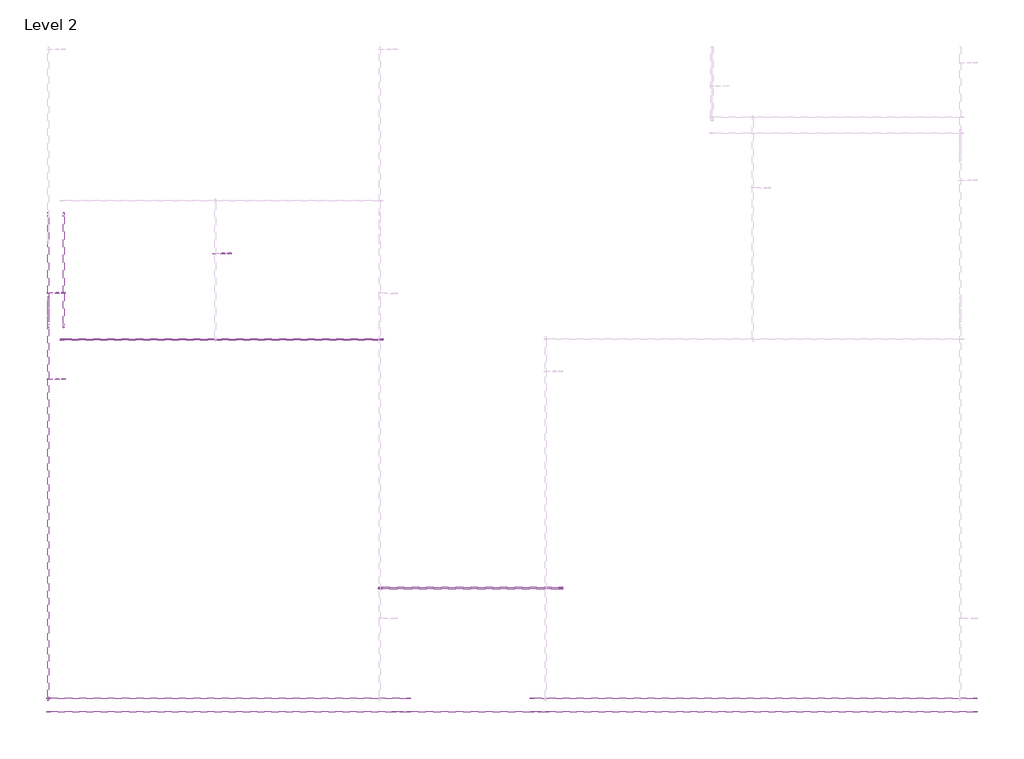
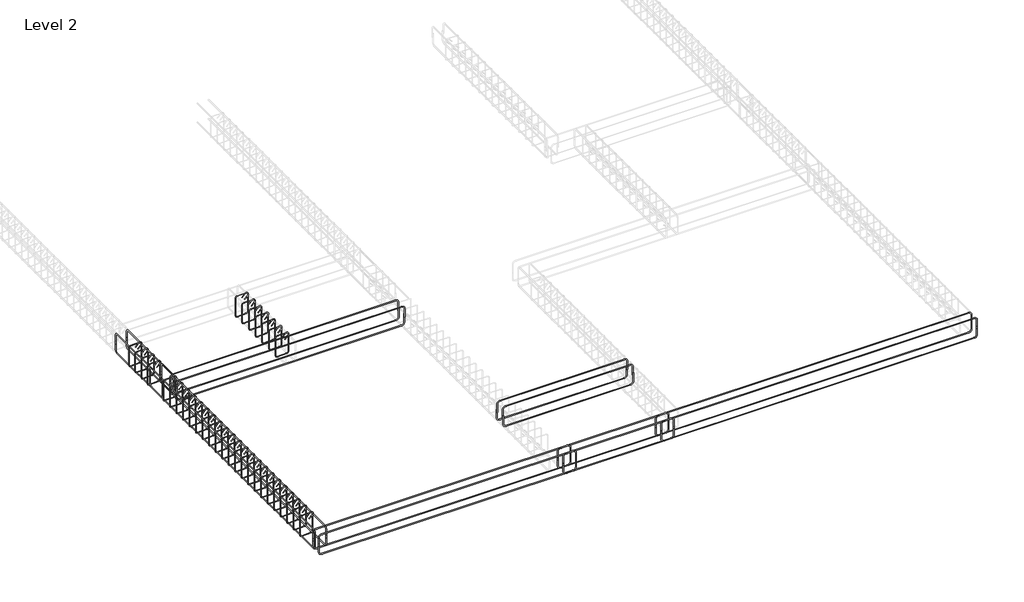
# One storey, part 2 of 5: 17 reinforcing bars.
"""IFC4 building model written with IfcOpenShell, lengths in millimetres."""

from ifc_helpers import new_model, si_unit, point, frame, origin, place, context, project, spatial, polyline, circle_curve, trimmed, segment, composite_curve, source, transform, mapped, element, save
from ifc_brep_helpers import swept_disk

model = new_model("IFC4")

# Units and contexts
model_context = context("Model", 3, world=origin())
ifc_project = project(units=[si_unit("LENGTHUNIT", "METRE", prefix="MILLI")], contexts=[model_context])

# Site, building, storey
site = spatial("IfcSite", under=ifc_project)
building = spatial("IfcBuilding", under=site)
storey = spatial("IfcBuildingStorey", under=building, Name="Level 2", Elevation=3048.0)

# Reinforcing bars
placement = place(None, origin())
reinforcing_bar_shape = source(origin(), model_context, "Body", "SolidModel", [
    swept_disk(composite_curve([segment(polyline([(-15212.455746, 3821.0577522, 5841.8967919), (-15212.455746, 3821.0577522, 5994.2967919)]), True, "CONTINUOUS"), segment(trimmed(circle_curve(frame((-15212.455746, 3776.9887522, 5994.2967919), z_axis=(1.0, 0.0, 0.0), x_axis=(0.0, 44.06899999999996, 0.0)), 44.069), [point((-15212.455746, 3821.0577522, 5994.2967919))], [point((-15212.455746, 3776.9887522, 6038.3657919))], True, "CARTESIAN"), True, "CONTINUOUS"), segment(polyline([(-15212.455746, 3776.9887522, 6038.3657919), (-15212.455746, 2478.6647522, 6038.3657919)]), True, "CONTINUOUS"), segment(trimmed(circle_curve(frame((-15212.455746, 2478.6647522, 5994.2967919), z_axis=(1.0, 0.0, 0.0), x_axis=(0.0, 0.0, 44.068999999999505)), 44.069), [point((-15212.455746, 2478.6647522, 6038.3657919))], [point((-15212.455746, 2434.5957522, 5994.2967919))], True, "CARTESIAN"), True, "CONTINUOUS"), segment(polyline([(-15212.455746, 2434.5957522, 5994.2967919), (-15212.455746, 2434.5957522, 5841.8967919)]), True, "CONTINUOUS")], self_intersect=False), 5.969),
])
element("IfcReinforcingBar", 1, at=placement, inside=storey, context=model_context, shape_type="MappedRepresentation", body=[
    mapped(reinforcing_bar_shape, transform((0.0, 0.0, 0.0), x_axis=(1.0, 0.0, 0.0), y_axis=(0.0, 1.0, 0.0), z_axis=(0.0, 0.0, 1.0))),
    mapped(reinforcing_bar_shape, transform((-189.5315837, 0.0, 0.0), x_axis=(1.0, 0.0, 0.0), y_axis=(0.0, 1.0, 0.0), z_axis=(0.0, 0.0, 1.0))),
])
reinforcing_bar_2_shape = source(origin(), model_context, "Body", "SolidModel", [
    swept_disk(composite_curve([segment(polyline([(-15212.455746, 2434.5957522, 5892.9032081), (-15212.455746, 2434.5957522, 5740.5032081)]), True, "CONTINUOUS"), segment(trimmed(circle_curve(frame((-15212.455746, 2478.6647522, 5740.5032081), z_axis=(1.0, 0.0, 0.0), x_axis=(0.0, -44.06899999999996, 0.0)), 44.069), [point((-15212.455746, 2434.5957522, 5740.5032081))], [point((-15212.455746, 2478.6647522, 5696.4342081))], True, "CARTESIAN"), True, "CONTINUOUS"), segment(polyline([(-15212.455746, 2478.6647522, 5696.4342081), (-15212.455746, 3776.9887522, 5696.4342081)]), True, "CONTINUOUS"), segment(trimmed(circle_curve(frame((-15212.455746, 3776.9887522, 5740.5032081), z_axis=(1.0, 0.0, 0.0), x_axis=(0.0, 0.0, -44.068999999999505)), 44.069), [point((-15212.455746, 3776.9887522, 5696.4342081))], [point((-15212.455746, 3821.0577522, 5740.5032081))], True, "CARTESIAN"), True, "CONTINUOUS"), segment(polyline([(-15212.455746, 3821.0577522, 5740.5032081), (-15212.455746, 3821.0577522, 5892.9032081)]), True, "CONTINUOUS")], self_intersect=False), 5.969),
])
element("IfcReinforcingBar", 2, at=placement, inside=storey, context=model_context, shape_type="MappedRepresentation", body=[
    mapped(reinforcing_bar_2_shape, transform((0.0, 0.0, 0.0), x_axis=(1.0, 0.0, 0.0), y_axis=(0.0, 1.0, 0.0), z_axis=(0.0, 0.0, 1.0))),
    mapped(reinforcing_bar_2_shape, transform((-189.5315837, 0.0, 0.0), x_axis=(1.0, 0.0, 0.0), y_axis=(0.0, 1.0, 0.0), z_axis=(0.0, 0.0, 1.0))),
])
reinforcing_bar_3_shape = source(origin(), model_context, "Body", "SolidModel", [
    swept_disk(composite_curve([segment(polyline([(-15212.455746, 2803.6577522, 5841.8967919), (-15212.455746, 2803.6577522, 5994.2967919)]), True, "CONTINUOUS"), segment(trimmed(circle_curve(frame((-15212.455746, 2759.5887522, 5994.2967919), z_axis=(1.0, 0.0, 0.0), x_axis=(0.0, 44.06899999999996, 0.0)), 44.069), [point((-15212.455746, 2803.6577522, 5994.2967919))], [point((-15212.455746, 2759.5887522, 6038.3657919))], True, "CARTESIAN"), True, "CONTINUOUS"), segment(polyline([(-15212.455746, 2759.5887522, 6038.3657919), (-15212.455746, -2021.3352478, 6038.3657919)]), True, "CONTINUOUS"), segment(trimmed(circle_curve(frame((-15212.455746, -2021.3352478, 5994.2967919), z_axis=(1.0, 0.0, 0.0), x_axis=(0.0, 0.0, 44.068999999999505)), 44.069), [point((-15212.455746, -2021.3352478, 6038.3657919))], [point((-15212.455746, -2065.4042478, 5994.2967919))], True, "CARTESIAN"), True, "CONTINUOUS"), segment(polyline([(-15212.455746, -2065.4042478, 5994.2967919), (-15212.455746, -2065.4042478, 5841.8967919)]), True, "CONTINUOUS")], self_intersect=False), 5.969),
])
element("IfcReinforcingBar", 3, at=placement, inside=storey, context=model_context, shape_type="MappedRepresentation", body=[
    mapped(reinforcing_bar_3_shape, transform((0.0, 0.0, 0.0), x_axis=(1.0, 0.0, 0.0), y_axis=(0.0, 1.0, 0.0), z_axis=(0.0, 0.0, 1.0))),
    mapped(reinforcing_bar_3_shape, transform((-189.5315837, 0.0, 0.0), x_axis=(1.0, 0.0, 0.0), y_axis=(0.0, 1.0, 0.0), z_axis=(0.0, 0.0, 1.0))),
])
reinforcing_bar_4_shape = source(origin(), model_context, "Body", "SolidModel", [
    swept_disk(composite_curve([segment(polyline([(-15212.455746, -2065.4042478, 5892.9032081), (-15212.455746, -2065.4042478, 5740.5032081)]), True, "CONTINUOUS"), segment(trimmed(circle_curve(frame((-15212.455746, -2021.3352478, 5740.5032081), z_axis=(1.0, 0.0, 0.0), x_axis=(0.0, -44.06900000000019, 0.0)), 44.069), [point((-15212.455746, -2065.4042478, 5740.5032081))], [point((-15212.455746, -2021.3352478, 5696.4342081))], True, "CARTESIAN"), True, "CONTINUOUS"), segment(polyline([(-15212.455746, -2021.3352478, 5696.4342081), (-15212.455746, 2759.5887522, 5696.4342081)]), True, "CONTINUOUS"), segment(trimmed(circle_curve(frame((-15212.455746, 2759.5887522, 5740.5032081), z_axis=(1.0, 0.0, 0.0), x_axis=(0.0, 0.0, -44.068999999999505)), 44.069), [point((-15212.455746, 2759.5887522, 5696.4342081))], [point((-15212.455746, 2803.6577522, 5740.5032081))], True, "CARTESIAN"), True, "CONTINUOUS"), segment(polyline([(-15212.455746, 2803.6577522, 5740.5032081), (-15212.455746, 2803.6577522, 5892.9032081)]), True, "CONTINUOUS")], self_intersect=False), 5.969),
])
element("IfcReinforcingBar", 4, at=placement, inside=storey, context=model_context, shape_type="MappedRepresentation", body=[
    mapped(reinforcing_bar_4_shape, transform((0.0, 0.0, 0.0), x_axis=(1.0, 0.0, 0.0), y_axis=(0.0, 1.0, 0.0), z_axis=(0.0, 0.0, 1.0))),
    mapped(reinforcing_bar_4_shape, transform((-189.5315837, 0.0, 0.0), x_axis=(1.0, 0.0, 0.0), y_axis=(0.0, 1.0, 0.0), z_axis=(0.0, 0.0, 1.0))),
])
reinforcing_bar_5_shape = source(origin(), model_context, "Body", "SolidModel", [
    swept_disk(composite_curve([segment(polyline([(-15260.3161447, 3403.9897522, 5949.0166099), (-15205.4511463, 3403.9897522, 6003.8816084)]), True, "CONTINUOUS"), segment(trimmed(circle_curve(frame((-15226.1955379, 3403.9897522, 6024.626), z_axis=(0.0, -1.0, 0.0), x_axis=(20.74439159999929, 0.0, -20.7443916000002)), 29.337), [point((-15205.4511463, 3403.9897522, 6003.8816084))], [point((-15226.1955379, 3403.9897522, 6053.963))], True, "CARTESIAN"), True, "CONTINUOUS"), segment(polyline([(-15226.1955379, 3403.9897522, 6053.963), (-15388.2475379, 3403.9897522, 6053.963)]), True, "CONTINUOUS"), segment(trimmed(circle_curve(frame((-15388.2475379, 3403.9897522, 6024.626), z_axis=(0.0, -1.0, 0.0), x_axis=(0.0, 0.0, 29.336999999999534)), 29.337), [point((-15388.2475379, 3403.9897522, 6053.963))], [point((-15417.5845379, 3403.9897522, 6024.626))], True, "CARTESIAN"), True, "CONTINUOUS"), segment(polyline([(-15417.5845379, 3403.9897522, 6024.626), (-15417.5845379, 3403.9897522, 5710.174)]), True, "CONTINUOUS"), segment(trimmed(circle_curve(frame((-15388.2661869, 3405.0356312, 5710.174), z_axis=(0.03565051078635061, -0.9993643184948482, 0.0), x_axis=(-29.318350999999893, -1.0458789999997862, 0.0)), 29.337), [point((-15417.5845379, 3403.9897522, 5710.174))], [point((-15388.2661869, 3405.0356312, 5680.837))], True, "CARTESIAN"), True, "CONTINUOUS"), segment(polyline([(-15388.2661869, 3405.0356312, 5680.837), (-15226.1768889, 3410.8178731, 5680.837)]), True, "CONTINUOUS"), segment(trimmed(circle_curve(frame((-15226.1768889, 3410.8178731, 5710.174), z_axis=(0.03565051078635061, -0.9993643184948482, 0.0), x_axis=(0.0, 0.0, -29.336999999999534)), 29.337), [point((-15226.1768889, 3410.8178731, 5680.837))], [point((-15196.8585379, 3411.8637522, 5710.174))], True, "CARTESIAN"), True, "CONTINUOUS"), segment(polyline([(-15196.8585379, 3411.8637522, 5710.174), (-15196.8585379, 3411.8637522, 6024.626)]), True, "CONTINUOUS"), segment(trimmed(circle_curve(frame((-15226.1955379, 3411.8637522, 6024.626), z_axis=(0.0, -1.0, 0.0), x_axis=(29.336999999999534, 0.0, 0.0)), 29.337), [point((-15196.8585379, 3411.8637522, 6024.626))], [point((-15246.9399295, 3411.8637522, 6045.3703916))], True, "CARTESIAN"), True, "CONTINUOUS"), segment(polyline([(-15246.9399295, 3411.8637522, 6045.3703916), (-15301.804928, 3411.8637522, 5990.5053932)]), True, "CONTINUOUS")], self_intersect=False), 3.937),
])
element("IfcReinforcingBar", 5, at=placement, inside=storey, context=model_context, shape_type="MappedRepresentation", body=[
    mapped(reinforcing_bar_5_shape, transform((0.0, 0.0, 0.0), x_axis=(1.0, 0.0, 0.0), y_axis=(0.0, 1.0, 0.0), z_axis=(0.0, 0.0, 1.0))),
    mapped(reinforcing_bar_5_shape, transform((0.0, -184.1086667, 0.0), x_axis=(1.0, 0.0, 0.0), y_axis=(0.0, 1.0, 0.0), z_axis=(0.0, 0.0, 1.0))),
    mapped(reinforcing_bar_5_shape, transform((0.0, -368.2173333, 0.0), x_axis=(1.0, 0.0, 0.0), y_axis=(0.0, 1.0, 0.0), z_axis=(0.0, 0.0, 1.0))),
    mapped(reinforcing_bar_5_shape, transform((0.0, -552.326, 0.0), x_axis=(1.0, 0.0, 0.0), y_axis=(0.0, 1.0, 0.0), z_axis=(0.0, 0.0, 1.0))),
])
reinforcing_bar_6_shape = source(origin(), model_context, "Body", "SolidModel", [
    swept_disk(composite_curve([segment(polyline([(-15260.3161447, 2386.5897522, 5949.0166099), (-15205.4511463, 2386.5897522, 6003.8816084)]), True, "CONTINUOUS"), segment(trimmed(circle_curve(frame((-15226.1955379, 2386.5897522, 6024.626), z_axis=(0.0, -1.0, 0.0), x_axis=(20.74439159999929, 0.0, -20.7443916000002)), 29.337), [point((-15205.4511463, 2386.5897522, 6003.8816084))], [point((-15226.1955379, 2386.5897522, 6053.963))], True, "CARTESIAN"), True, "CONTINUOUS"), segment(polyline([(-15226.1955379, 2386.5897522, 6053.963), (-15388.2475379, 2386.5897522, 6053.963)]), True, "CONTINUOUS"), segment(trimmed(circle_curve(frame((-15388.2475379, 2386.5897522, 6024.626), z_axis=(0.0, -1.0, 0.0), x_axis=(0.0, 0.0, 29.336999999999534)), 29.337), [point((-15388.2475379, 2386.5897522, 6053.963))], [point((-15417.5845379, 2386.5897522, 6024.626))], True, "CARTESIAN"), True, "CONTINUOUS"), segment(polyline([(-15417.5845379, 2386.5897522, 6024.626), (-15417.5845379, 2386.5897522, 5710.174)]), True, "CONTINUOUS"), segment(trimmed(circle_curve(frame((-15388.2661869, 2387.6356312, 5710.174), z_axis=(0.03565051078634999, -0.9993643184948483, 0.0), x_axis=(-29.318350999999893, -1.0458789999997862, 0.0)), 29.337), [point((-15417.5845379, 2386.5897522, 5710.174))], [point((-15388.2661869, 2387.6356312, 5680.837))], True, "CARTESIAN"), True, "CONTINUOUS"), segment(polyline([(-15388.2661869, 2387.6356312, 5680.837), (-15226.1768889, 2393.4178731, 5680.837)]), True, "CONTINUOUS"), segment(trimmed(circle_curve(frame((-15226.1768889, 2393.4178731, 5710.174), z_axis=(0.03565051078634999, -0.9993643184948483, 0.0), x_axis=(0.0, 0.0, -29.336999999999534)), 29.337), [point((-15226.1768889, 2393.4178731, 5680.837))], [point((-15196.8585379, 2394.4637522, 5710.174))], True, "CARTESIAN"), True, "CONTINUOUS"), segment(polyline([(-15196.8585379, 2394.4637522, 5710.174), (-15196.8585379, 2394.4637522, 6024.626)]), True, "CONTINUOUS"), segment(trimmed(circle_curve(frame((-15226.1955379, 2394.4637522, 6024.626), z_axis=(0.0, -1.0, 0.0), x_axis=(29.336999999999534, 0.0, 0.0)), 29.337), [point((-15196.8585379, 2394.4637522, 6024.626))], [point((-15246.9399295, 2394.4637522, 6045.3703916))], True, "CARTESIAN"), True, "CONTINUOUS"), segment(polyline([(-15246.9399295, 2394.4637522, 6045.3703916), (-15301.804928, 2394.4637522, 5990.5053932)]), True, "CONTINUOUS")], self_intersect=False), 3.937),
])
element("IfcReinforcingBar", 6, at=placement, inside=storey, context=model_context, shape_type="MappedRepresentation", body=[
    mapped(reinforcing_bar_6_shape, transform((0.0, 0.0, 0.0), x_axis=(1.0, 0.0, 0.0), y_axis=(0.0, 1.0, 0.0), z_axis=(0.0, 0.0, 1.0))),
    mapped(reinforcing_bar_6_shape, transform((0.0, -192.1393333, 0.0), x_axis=(1.0, 0.0, 0.0), y_axis=(0.0, 1.0, 0.0), z_axis=(0.0, 0.0, 1.0))),
    mapped(reinforcing_bar_6_shape, transform((0.0, -384.2786667, 0.0), x_axis=(1.0, 0.0, 0.0), y_axis=(0.0, 1.0, 0.0), z_axis=(0.0, 0.0, 1.0))),
    mapped(reinforcing_bar_6_shape, transform((0.0, -576.418, 0.0), x_axis=(1.0, 0.0, 0.0), y_axis=(0.0, 1.0, 0.0), z_axis=(0.0, 0.0, 1.0))),
    mapped(reinforcing_bar_6_shape, transform((0.0, -768.5573333, 0.0), x_axis=(1.0, 0.0, 0.0), y_axis=(0.0, 1.0, 0.0), z_axis=(0.0, 0.0, 1.0))),
    mapped(reinforcing_bar_6_shape, transform((0.0, -960.6966667, 0.0), x_axis=(1.0, 0.0, 0.0), y_axis=(0.0, 1.0, 0.0), z_axis=(0.0, 0.0, 1.0))),
    mapped(reinforcing_bar_6_shape, transform((0.0, -1152.836, 0.0), x_axis=(1.0, 0.0, 0.0), y_axis=(0.0, 1.0, 0.0), z_axis=(0.0, 0.0, 1.0))),
    mapped(reinforcing_bar_6_shape, transform((0.0, -1344.9753333, 0.0), x_axis=(1.0, 0.0, 0.0), y_axis=(0.0, 1.0, 0.0), z_axis=(0.0, 0.0, 1.0))),
    mapped(reinforcing_bar_6_shape, transform((0.0, -1537.1146667, 0.0), x_axis=(1.0, 0.0, 0.0), y_axis=(0.0, 1.0, 0.0), z_axis=(0.0, 0.0, 1.0))),
    mapped(reinforcing_bar_6_shape, transform((0.0, -1729.254, 0.0), x_axis=(1.0, 0.0, 0.0), y_axis=(0.0, 1.0, 0.0), z_axis=(0.0, 0.0, 1.0))),
    mapped(reinforcing_bar_6_shape, transform((0.0, -1921.3933333, 0.0), x_axis=(1.0, 0.0, 0.0), y_axis=(0.0, 1.0, 0.0), z_axis=(0.0, 0.0, 1.0))),
    mapped(reinforcing_bar_6_shape, transform((0.0, -2113.5326667, 0.0), x_axis=(1.0, 0.0, 0.0), y_axis=(0.0, 1.0, 0.0), z_axis=(0.0, 0.0, 1.0))),
    mapped(reinforcing_bar_6_shape, transform((0.0, -2305.672, 0.0), x_axis=(1.0, 0.0, 0.0), y_axis=(0.0, 1.0, 0.0), z_axis=(0.0, 0.0, 1.0))),
    mapped(reinforcing_bar_6_shape, transform((0.0, -2497.8113333, 0.0), x_axis=(1.0, 0.0, 0.0), y_axis=(0.0, 1.0, 0.0), z_axis=(0.0, 0.0, 1.0))),
    mapped(reinforcing_bar_6_shape, transform((0.0, -2689.9506667, 0.0), x_axis=(1.0, 0.0, 0.0), y_axis=(0.0, 1.0, 0.0), z_axis=(0.0, 0.0, 1.0))),
    mapped(reinforcing_bar_6_shape, transform((0.0, -2882.09, 0.0), x_axis=(1.0, 0.0, 0.0), y_axis=(0.0, 1.0, 0.0), z_axis=(0.0, 0.0, 1.0))),
    mapped(reinforcing_bar_6_shape, transform((0.0, -3074.2293333, 0.0), x_axis=(1.0, 0.0, 0.0), y_axis=(0.0, 1.0, 0.0), z_axis=(0.0, 0.0, 1.0))),
    mapped(reinforcing_bar_6_shape, transform((0.0, -3266.3686667, 0.0), x_axis=(1.0, 0.0, 0.0), y_axis=(0.0, 1.0, 0.0), z_axis=(0.0, 0.0, 1.0))),
    mapped(reinforcing_bar_6_shape, transform((0.0, -3458.508, 0.0), x_axis=(1.0, 0.0, 0.0), y_axis=(0.0, 1.0, 0.0), z_axis=(0.0, 0.0, 1.0))),
    mapped(reinforcing_bar_6_shape, transform((0.0, -3650.6473333, 0.0), x_axis=(1.0, 0.0, 0.0), y_axis=(0.0, 1.0, 0.0), z_axis=(0.0, 0.0, 1.0))),
    mapped(reinforcing_bar_6_shape, transform((0.0, -3842.7866667, 0.0), x_axis=(1.0, 0.0, 0.0), y_axis=(0.0, 1.0, 0.0), z_axis=(0.0, 0.0, 1.0))),
    mapped(reinforcing_bar_6_shape, transform((0.0, -4034.926, 0.0), x_axis=(1.0, 0.0, 0.0), y_axis=(0.0, 1.0, 0.0), z_axis=(0.0, 0.0, 1.0))),
])
reinforcing_bar_7_shape = source(origin(), model_context, "Body", "SolidModel", [
    swept_disk(composite_curve([segment(polyline([(-13260.3161447, 3721.4897522, 5949.0166099), (-13205.4511463, 3721.4897522, 6003.8816084)]), True, "CONTINUOUS"), segment(trimmed(circle_curve(frame((-13226.1955379, 3721.4897522, 6024.626), z_axis=(0.0, -1.0, 0.0), x_axis=(20.74439159999929, 0.0, -20.7443916000002)), 29.337), [point((-13205.4511463, 3721.4897522, 6003.8816084))], [point((-13226.1955379, 3721.4897522, 6053.963))], True, "CARTESIAN"), True, "CONTINUOUS"), segment(polyline([(-13226.1955379, 3721.4897522, 6053.963), (-13388.2475379, 3721.4897522, 6053.963)]), True, "CONTINUOUS"), segment(trimmed(circle_curve(frame((-13388.2475379, 3721.4897522, 6024.626), z_axis=(0.0, -1.0, 0.0), x_axis=(0.0, 0.0, 29.336999999999534)), 29.337), [point((-13388.2475379, 3721.4897522, 6053.963))], [point((-13417.5845379, 3721.4897522, 6024.626))], True, "CARTESIAN"), True, "CONTINUOUS"), segment(polyline([(-13417.5845379, 3721.4897522, 6024.626), (-13417.5845379, 3721.4897522, 5710.174)]), True, "CONTINUOUS"), segment(trimmed(circle_curve(frame((-13388.2661869, 3722.5356312, 5710.174), z_axis=(0.035650510786350516, -0.9993643184948482, 0.0), x_axis=(-29.318350999999893, -1.0458789999997862, 0.0)), 29.337), [point((-13417.5845379, 3721.4897522, 5710.174))], [point((-13388.2661869, 3722.5356312, 5680.837))], True, "CARTESIAN"), True, "CONTINUOUS"), segment(polyline([(-13388.2661869, 3722.5356312, 5680.837), (-13226.1768889, 3728.3178731, 5680.837)]), True, "CONTINUOUS"), segment(trimmed(circle_curve(frame((-13226.1768889, 3728.3178731, 5710.174), z_axis=(0.035650510786350516, -0.9993643184948482, 0.0), x_axis=(0.0, 0.0, -29.336999999999534)), 29.337), [point((-13226.1768889, 3728.3178731, 5680.837))], [point((-13196.8585379, 3729.3637522, 5710.174))], True, "CARTESIAN"), True, "CONTINUOUS"), segment(polyline([(-13196.8585379, 3729.3637522, 5710.174), (-13196.8585379, 3729.3637522, 6024.626)]), True, "CONTINUOUS"), segment(trimmed(circle_curve(frame((-13226.1955379, 3729.3637522, 6024.626), z_axis=(0.0, -1.0, 0.0), x_axis=(29.336999999999534, 0.0, 0.0)), 29.337), [point((-13196.8585379, 3729.3637522, 6024.626))], [point((-13246.9399295, 3729.3637522, 6045.3703916))], True, "CARTESIAN"), True, "CONTINUOUS"), segment(polyline([(-13246.9399295, 3729.3637522, 6045.3703916), (-13301.804928, 3729.3637522, 5990.5053932)]), True, "CONTINUOUS")], self_intersect=False), 3.937),
])
element("IfcReinforcingBar", 7, at=placement, inside=storey, context=model_context, shape_type="MappedRepresentation", body=[
    mapped(reinforcing_bar_7_shape, transform((0.0, 0.0, 0.0), x_axis=(1.0, 0.0, 0.0), y_axis=(0.0, 1.0, 0.0), z_axis=(0.0, 0.0, 1.0))),
    mapped(reinforcing_bar_7_shape, transform((0.0, -197.8876667, 0.0), x_axis=(1.0, 0.0, 0.0), y_axis=(0.0, 1.0, 0.0), z_axis=(0.0, 0.0, 1.0))),
    mapped(reinforcing_bar_7_shape, transform((0.0, -395.7753333, 0.0), x_axis=(1.0, 0.0, 0.0), y_axis=(0.0, 1.0, 0.0), z_axis=(0.0, 0.0, 1.0))),
    mapped(reinforcing_bar_7_shape, transform((0.0, -593.663, 0.0), x_axis=(1.0, 0.0, 0.0), y_axis=(0.0, 1.0, 0.0), z_axis=(0.0, 0.0, 1.0))),
    mapped(reinforcing_bar_7_shape, transform((0.0, -791.5506667, 0.0), x_axis=(1.0, 0.0, 0.0), y_axis=(0.0, 1.0, 0.0), z_axis=(0.0, 0.0, 1.0))),
    mapped(reinforcing_bar_7_shape, transform((0.0, -989.4383333, 0.0), x_axis=(1.0, 0.0, 0.0), y_axis=(0.0, 1.0, 0.0), z_axis=(0.0, 0.0, 1.0))),
    mapped(reinforcing_bar_7_shape, transform((0.0, -1187.326, 0.0), x_axis=(1.0, 0.0, 0.0), y_axis=(0.0, 1.0, 0.0), z_axis=(0.0, 0.0, 1.0))),
])
reinforcing_bar_8_shape = source(origin(), model_context, "Body", "SolidModel", [
    swept_disk(composite_curve([segment(polyline([(-11363.9905379, 2283.0609603, 5841.8967919), (-11363.9905379, 2283.0609603, 5994.2967919)]), True, "CONTINUOUS"), segment(trimmed(circle_curve(frame((-11408.0595379, 2283.0609603, 5994.2967919), z_axis=(0.0, -1.0, 0.0), x_axis=(44.069000000001324, 0.0, 0.0)), 44.069), [point((-11363.9905379, 2283.0609603, 5994.2967919))], [point((-11408.0595379, 2283.0609603, 6038.3657919))], True, "CARTESIAN"), True, "CONTINUOUS"), segment(polyline([(-11408.0595379, 2283.0609603, 6038.3657919), (-15206.3835379, 2283.0609603, 6038.3657919)]), True, "CONTINUOUS"), segment(trimmed(circle_curve(frame((-15206.3835379, 2283.0609603, 5994.2967919), z_axis=(0.0, -1.0, 0.0), x_axis=(0.0, 0.0, 44.068999999999505)), 44.069), [point((-15206.3835379, 2283.0609603, 6038.3657919))], [point((-15250.4525379, 2283.0609603, 5994.2967919))], True, "CARTESIAN"), True, "CONTINUOUS"), segment(polyline([(-15250.4525379, 2283.0609603, 5994.2967919), (-15250.4525379, 2283.0609603, 5841.8967919)]), True, "CONTINUOUS")], self_intersect=False), 5.969),
])
element("IfcReinforcingBar", 8, at=placement, inside=storey, context=model_context, shape_type="MappedRepresentation", body=[
    mapped(reinforcing_bar_8_shape, transform((0.0, 0.0, 0.0), x_axis=(1.0, 0.0, 0.0), y_axis=(0.0, 1.0, 0.0), z_axis=(0.0, 0.0, 1.0))),
    mapped(reinforcing_bar_8_shape, transform((0.0, 189.5315837, 0.0), x_axis=(1.0, 0.0, 0.0), y_axis=(0.0, 1.0, 0.0), z_axis=(0.0, 0.0, 1.0))),
])
reinforcing_bar_9_shape = source(origin(), model_context, "Body", "SolidModel", [
    swept_disk(composite_curve([segment(polyline([(-15250.4525379, 2458.8527522, 5887.212), (-15250.4525379, 2458.8527522, 5734.812)]), True, "CONTINUOUS"), segment(trimmed(circle_curve(frame((-15206.3835379, 2458.8527522, 5734.812), z_axis=(0.0, -1.0, 0.0), x_axis=(-44.069000000001324, 0.0, 0.0)), 44.069), [point((-15250.4525379, 2458.8527522, 5734.812))], [point((-15206.3835379, 2458.8527522, 5690.743))], True, "CARTESIAN"), True, "CONTINUOUS"), segment(polyline([(-15206.3835379, 2458.8527522, 5690.743), (-11408.0595379, 2458.8527522, 5690.743)]), True, "CONTINUOUS"), segment(trimmed(circle_curve(frame((-11408.0595379, 2458.8527522, 5734.812), z_axis=(0.0, -1.0, 0.0), x_axis=(0.0, 0.0, -44.068999999999505)), 44.069), [point((-11408.0595379, 2458.8527522, 5690.743))], [point((-11363.9905379, 2458.8527522, 5734.812))], True, "CARTESIAN"), True, "CONTINUOUS"), segment(polyline([(-11363.9905379, 2458.8527522, 5734.812), (-11363.9905379, 2458.8527522, 5887.212)]), True, "CONTINUOUS")], self_intersect=False), 5.969),
])
element("IfcReinforcingBar", 9, at=placement, inside=storey, context=model_context, shape_type="MappedRepresentation", body=[
    mapped(reinforcing_bar_9_shape, transform((0.0, 0.0, 0.0), x_axis=(1.0, 0.0, 0.0), y_axis=(0.0, 1.0, 0.0), z_axis=(0.0, 0.0, 1.0))),
    mapped(reinforcing_bar_9_shape, transform((0.0, -162.052, 0.0), x_axis=(1.0, 0.0, 0.0), y_axis=(0.0, 1.0, 0.0), z_axis=(0.0, 0.0, 1.0))),
])
reinforcing_bar_10_shape = source(origin(), model_context, "Body", "SolidModel", [
    swept_disk(composite_curve([segment(polyline([(-9198.8905379, -541.1472478, 5847.588), (-9198.8905379, -541.1472478, 5999.988)]), True, "CONTINUOUS"), segment(trimmed(circle_curve(frame((-9242.9595379, -541.1472478, 5999.988), z_axis=(0.0, -1.0, 0.0), x_axis=(44.068999999999505, 0.0, 0.0)), 44.069), [point((-9198.8905379, -541.1472478, 5999.988))], [point((-9242.9595379, -541.1472478, 6044.057))], True, "CARTESIAN"), True, "CONTINUOUS"), segment(polyline([(-9242.9595379, -541.1472478, 6044.057), (-11371.4835379, -541.1472478, 6044.057)]), True, "CONTINUOUS"), segment(trimmed(circle_curve(frame((-11371.4835379, -541.1472478, 5999.988), z_axis=(0.0, -1.0, 0.0), x_axis=(0.0, 0.0, 44.068999999999505)), 44.069), [point((-11371.4835379, -541.1472478, 6044.057))], [point((-11415.5525379, -541.1472478, 5999.988))], True, "CARTESIAN"), True, "CONTINUOUS"), segment(polyline([(-11415.5525379, -541.1472478, 5999.988), (-11415.5525379, -541.1472478, 5847.588)]), True, "CONTINUOUS")], self_intersect=False), 5.969),
])
element("IfcReinforcingBar", 10, at=placement, inside=storey, context=model_context, shape_type="MappedRepresentation", body=[
    mapped(reinforcing_bar_10_shape, transform((0.0, 0.0, 0.0), x_axis=(1.0, 0.0, 0.0), y_axis=(0.0, 1.0, 0.0), z_axis=(0.0, 0.0, 1.0))),
    mapped(reinforcing_bar_10_shape, transform((0.0, -162.052, 0.0), x_axis=(1.0, 0.0, 0.0), y_axis=(0.0, 1.0, 0.0), z_axis=(0.0, 0.0, 1.0))),
])
reinforcing_bar_11_shape = source(origin(), model_context, "Body", "SolidModel", [
    swept_disk(composite_curve([segment(polyline([(-11415.5525379, -716.9390397, 5892.9032081), (-11415.5525379, -716.9390397, 5740.5032081)]), True, "CONTINUOUS"), segment(trimmed(circle_curve(frame((-11371.4835379, -716.9390397, 5740.5032081), z_axis=(0.0, -1.0, 0.0), x_axis=(-44.068999999999505, 0.0, 0.0)), 44.069), [point((-11415.5525379, -716.9390397, 5740.5032081))], [point((-11371.4835379, -716.9390397, 5696.4342081))], True, "CARTESIAN"), True, "CONTINUOUS"), segment(polyline([(-11371.4835379, -716.9390397, 5696.4342081), (-9242.9595379, -716.9390397, 5696.4342081)]), True, "CONTINUOUS"), segment(trimmed(circle_curve(frame((-9242.9595379, -716.9390397, 5740.5032081), z_axis=(0.0, -1.0, 0.0), x_axis=(0.0, 0.0, -44.068999999999505)), 44.069), [point((-9242.9595379, -716.9390397, 5696.4342081))], [point((-9198.8905379, -716.9390397, 5740.5032081))], True, "CARTESIAN"), True, "CONTINUOUS"), segment(polyline([(-9198.8905379, -716.9390397, 5740.5032081), (-9198.8905379, -716.9390397, 5892.9032081)]), True, "CONTINUOUS")], self_intersect=False), 5.969),
])
element("IfcReinforcingBar", 11, at=placement, inside=storey, context=model_context, shape_type="MappedRepresentation", body=[
    mapped(reinforcing_bar_11_shape, transform((0.0, 0.0, 0.0), x_axis=(1.0, 0.0, 0.0), y_axis=(0.0, 1.0, 0.0), z_axis=(0.0, 0.0, 1.0))),
    mapped(reinforcing_bar_11_shape, transform((0.0, 189.5315837, 0.0), x_axis=(1.0, 0.0, 0.0), y_axis=(0.0, 1.0, 0.0), z_axis=(0.0, 0.0, 1.0))),
])
reinforcing_bar_12_shape = source(origin(), model_context, "Body", "SolidModel", [
    swept_disk(composite_curve([segment(polyline([(-4198.8905379, -2041.1472478, 5847.588), (-4198.8905379, -2041.1472478, 5999.988)]), True, "CONTINUOUS"), segment(trimmed(circle_curve(frame((-4242.9595379, -2041.1472478, 5999.988), z_axis=(0.0, -1.0, 0.0), x_axis=(44.069000000000415, 0.0, 0.0)), 44.069), [point((-4198.8905379, -2041.1472478, 5999.988))], [point((-4242.9595379, -2041.1472478, 6044.057))], True, "CARTESIAN"), True, "CONTINUOUS"), segment(polyline([(-4242.9595379, -2041.1472478, 6044.057), (-9536.5835379, -2041.1472478, 6044.057)]), True, "CONTINUOUS"), segment(trimmed(circle_curve(frame((-9536.5835379, -2041.1472478, 5999.988), z_axis=(0.0, -1.0, 0.0), x_axis=(0.0, 0.0, 44.068999999999505)), 44.069), [point((-9536.5835379, -2041.1472478, 6044.057))], [point((-9580.6525379, -2041.1472478, 5999.988))], True, "CARTESIAN"), True, "CONTINUOUS"), segment(polyline([(-9580.6525379, -2041.1472478, 5999.988), (-9580.6525379, -2041.1472478, 5847.588)]), True, "CONTINUOUS")], self_intersect=False), 5.969),
])
element("IfcReinforcingBar", 12, at=placement, inside=storey, context=model_context, shape_type="MappedRepresentation", body=[
    mapped(reinforcing_bar_12_shape, transform((0.0, 0.0, 0.0), x_axis=(1.0, 0.0, 0.0), y_axis=(0.0, 1.0, 0.0), z_axis=(0.0, 0.0, 1.0))),
    mapped(reinforcing_bar_12_shape, transform((0.0, -162.052, 0.0), x_axis=(1.0, 0.0, 0.0), y_axis=(0.0, 1.0, 0.0), z_axis=(0.0, 0.0, 1.0))),
])
reinforcing_bar_13_shape = source(origin(), model_context, "Body", "SolidModel", [
    swept_disk(composite_curve([segment(polyline([(-9580.6525379, -2203.1992478, 5887.212), (-9580.6525379, -2203.1992478, 5734.812)]), True, "CONTINUOUS"), segment(trimmed(circle_curve(frame((-9536.5835379, -2203.1992478, 5734.812), z_axis=(0.0, -1.0, 0.0), x_axis=(-44.068999999999505, 0.0, 0.0)), 44.069), [point((-9580.6525379, -2203.1992478, 5734.812))], [point((-9536.5835379, -2203.1992478, 5690.743))], True, "CARTESIAN"), True, "CONTINUOUS"), segment(polyline([(-9536.5835379, -2203.1992478, 5690.743), (-4242.9595379, -2203.1992478, 5690.743)]), True, "CONTINUOUS"), segment(trimmed(circle_curve(frame((-4242.9595379, -2203.1992478, 5734.812), z_axis=(0.0, -1.0, 0.0), x_axis=(0.0, 0.0, -44.068999999999505)), 44.069), [point((-4242.9595379, -2203.1992478, 5690.743))], [point((-4198.8905379, -2203.1992478, 5734.812))], True, "CARTESIAN"), True, "CONTINUOUS"), segment(polyline([(-4198.8905379, -2203.1992478, 5734.812), (-4198.8905379, -2203.1992478, 5887.212)]), True, "CONTINUOUS")], self_intersect=False), 5.969),
])
element("IfcReinforcingBar", 13, at=placement, inside=storey, context=model_context, shape_type="MappedRepresentation", body=[
    mapped(reinforcing_bar_13_shape, transform((0.0, 0.0, 0.0), x_axis=(1.0, 0.0, 0.0), y_axis=(0.0, 1.0, 0.0), z_axis=(0.0, 0.0, 1.0))),
    mapped(reinforcing_bar_13_shape, transform((0.0, 162.052, 0.0), x_axis=(1.0, 0.0, 0.0), y_axis=(0.0, 1.0, 0.0), z_axis=(0.0, 0.0, 1.0))),
])
reinforcing_bar_14_shape = source(origin(), model_context, "Body", "SolidModel", [
    swept_disk(composite_curve([segment(polyline([(-9363.9905379, -2041.1472478, 5847.588), (-9363.9905379, -2041.1472478, 5999.988)]), True, "CONTINUOUS"), segment(trimmed(circle_curve(frame((-9408.0595379, -2041.1472478, 5999.988), z_axis=(0.0, -1.0, 0.0), x_axis=(44.069000000001324, 0.0, 0.0)), 44.069), [point((-9363.9905379, -2041.1472478, 5999.988))], [point((-9408.0595379, -2041.1472478, 6044.057))], True, "CARTESIAN"), True, "CONTINUOUS"), segment(polyline([(-9408.0595379, -2041.1472478, 6044.057), (-11206.3835379, -2041.1472478, 6044.057)]), True, "CONTINUOUS"), segment(trimmed(circle_curve(frame((-11206.3835379, -2041.1472478, 5999.988), z_axis=(0.0, -1.0, 0.0), x_axis=(0.0, 0.0, 44.068999999999505)), 44.069), [point((-11206.3835379, -2041.1472478, 6044.057))], [point((-11250.4525379, -2041.1472478, 5999.988))], True, "CARTESIAN"), True, "CONTINUOUS"), segment(polyline([(-11250.4525379, -2041.1472478, 5999.988), (-11250.4525379, -2041.1472478, 5847.588)]), True, "CONTINUOUS")], self_intersect=False), 5.969),
])
element("IfcReinforcingBar", 14, at=placement, inside=storey, context=model_context, shape_type="MappedRepresentation", body=[
    mapped(reinforcing_bar_14_shape, transform((0.0, 0.0, 0.0), x_axis=(1.0, 0.0, 0.0), y_axis=(0.0, 1.0, 0.0), z_axis=(0.0, 0.0, 1.0))),
    mapped(reinforcing_bar_14_shape, transform((0.0, -162.052, 0.0), x_axis=(1.0, 0.0, 0.0), y_axis=(0.0, 1.0, 0.0), z_axis=(0.0, 0.0, 1.0))),
])
reinforcing_bar_15_shape = source(origin(), model_context, "Body", "SolidModel", [
    swept_disk(composite_curve([segment(polyline([(-11250.4525379, -2203.1992478, 5887.212), (-11250.4525379, -2203.1992478, 5734.812)]), True, "CONTINUOUS"), segment(trimmed(circle_curve(frame((-11206.3835379, -2203.1992478, 5734.812), z_axis=(0.0, -1.0, 0.0), x_axis=(-44.069000000001324, 0.0, 0.0)), 44.069), [point((-11250.4525379, -2203.1992478, 5734.812))], [point((-11206.3835379, -2203.1992478, 5690.743))], True, "CARTESIAN"), True, "CONTINUOUS"), segment(polyline([(-11206.3835379, -2203.1992478, 5690.743), (-9408.0595379, -2203.1992478, 5690.743)]), True, "CONTINUOUS"), segment(trimmed(circle_curve(frame((-9408.0595379, -2203.1992478, 5734.812), z_axis=(0.0, -1.0, 0.0), x_axis=(0.0, 0.0, -44.068999999999505)), 44.069), [point((-9408.0595379, -2203.1992478, 5690.743))], [point((-9363.9905379, -2203.1992478, 5734.812))], True, "CARTESIAN"), True, "CONTINUOUS"), segment(polyline([(-9363.9905379, -2203.1992478, 5734.812), (-9363.9905379, -2203.1992478, 5887.212)]), True, "CONTINUOUS")], self_intersect=False), 5.969),
])
element("IfcReinforcingBar", 15, at=placement, inside=storey, context=model_context, shape_type="MappedRepresentation", body=[
    mapped(reinforcing_bar_15_shape, transform((0.0, 0.0, 0.0), x_axis=(1.0, 0.0, 0.0), y_axis=(0.0, 1.0, 0.0), z_axis=(0.0, 0.0, 1.0))),
    mapped(reinforcing_bar_15_shape, transform((0.0, 162.052, 0.0), x_axis=(1.0, 0.0, 0.0), y_axis=(0.0, 1.0, 0.0), z_axis=(0.0, 0.0, 1.0))),
])
reinforcing_bar_16_shape = source(origin(), model_context, "Body", "SolidModel", [
    swept_disk(composite_curve([segment(polyline([(-11033.7905379, -2041.1472478, 5847.588), (-11033.7905379, -2041.1472478, 5999.988)]), True, "CONTINUOUS"), segment(trimmed(circle_curve(frame((-11077.8595379, -2041.1472478, 5999.988), z_axis=(0.0, -1.0, 0.0), x_axis=(44.068999999999505, 0.0, 0.0)), 44.069), [point((-11033.7905379, -2041.1472478, 5999.988))], [point((-11077.8595379, -2041.1472478, 6044.057))], True, "CARTESIAN"), True, "CONTINUOUS"), segment(polyline([(-11077.8595379, -2041.1472478, 6044.057), (-15371.4835379, -2041.1472478, 6044.057)]), True, "CONTINUOUS"), segment(trimmed(circle_curve(frame((-15371.4835379, -2041.1472478, 5999.988), z_axis=(0.0, -1.0, 0.0), x_axis=(0.0, 0.0, 44.068999999999505)), 44.069), [point((-15371.4835379, -2041.1472478, 6044.057))], [point((-15415.5525379, -2041.1472478, 5999.988))], True, "CARTESIAN"), True, "CONTINUOUS"), segment(polyline([(-15415.5525379, -2041.1472478, 5999.988), (-15415.5525379, -2041.1472478, 5847.588)]), True, "CONTINUOUS")], self_intersect=False), 5.969),
])
element("IfcReinforcingBar", 16, at=placement, inside=storey, context=model_context, shape_type="MappedRepresentation", body=[
    mapped(reinforcing_bar_16_shape, transform((0.0, 0.0, 0.0), x_axis=(1.0, 0.0, 0.0), y_axis=(0.0, 1.0, 0.0), z_axis=(0.0, 0.0, 1.0))),
    mapped(reinforcing_bar_16_shape, transform((0.0, -162.052, 0.0), x_axis=(1.0, 0.0, 0.0), y_axis=(0.0, 1.0, 0.0), z_axis=(0.0, 0.0, 1.0))),
])
reinforcing_bar_17_shape = source(origin(), model_context, "Body", "SolidModel", [
    swept_disk(composite_curve([segment(polyline([(-15415.5525379, -2203.1992478, 5887.212), (-15415.5525379, -2203.1992478, 5734.812)]), True, "CONTINUOUS"), segment(trimmed(circle_curve(frame((-15371.4835379, -2203.1992478, 5734.812), z_axis=(0.0, -1.0, 0.0), x_axis=(-44.068999999999505, 0.0, 0.0)), 44.069), [point((-15415.5525379, -2203.1992478, 5734.812))], [point((-15371.4835379, -2203.1992478, 5690.743))], True, "CARTESIAN"), True, "CONTINUOUS"), segment(polyline([(-15371.4835379, -2203.1992478, 5690.743), (-11077.8595379, -2203.1992478, 5690.743)]), True, "CONTINUOUS"), segment(trimmed(circle_curve(frame((-11077.8595379, -2203.1992478, 5734.812), z_axis=(0.0, -1.0, 0.0), x_axis=(0.0, 0.0, -44.068999999999505)), 44.069), [point((-11077.8595379, -2203.1992478, 5690.743))], [point((-11033.7905379, -2203.1992478, 5734.812))], True, "CARTESIAN"), True, "CONTINUOUS"), segment(polyline([(-11033.7905379, -2203.1992478, 5734.812), (-11033.7905379, -2203.1992478, 5887.212)]), True, "CONTINUOUS")], self_intersect=False), 5.969),
])
element("IfcReinforcingBar", 17, at=placement, inside=storey, context=model_context, shape_type="MappedRepresentation", body=[
    mapped(reinforcing_bar_17_shape, transform((0.0, 0.0, 0.0), x_axis=(1.0, 0.0, 0.0), y_axis=(0.0, 1.0, 0.0), z_axis=(0.0, 0.0, 1.0))),
    mapped(reinforcing_bar_17_shape, transform((0.0, 162.052, 0.0), x_axis=(1.0, 0.0, 0.0), y_axis=(0.0, 1.0, 0.0), z_axis=(0.0, 0.0, 1.0))),
])

save(model, "model.ifc")

# Revit data of these elements
# Elements 1, 2, 3, 4, 5, 6, 7, 8, 9, 10, 11, 12, 13, 14, 15, 16, 17 (IfcReinforcingBar)
#   Phase Created = New Construction
